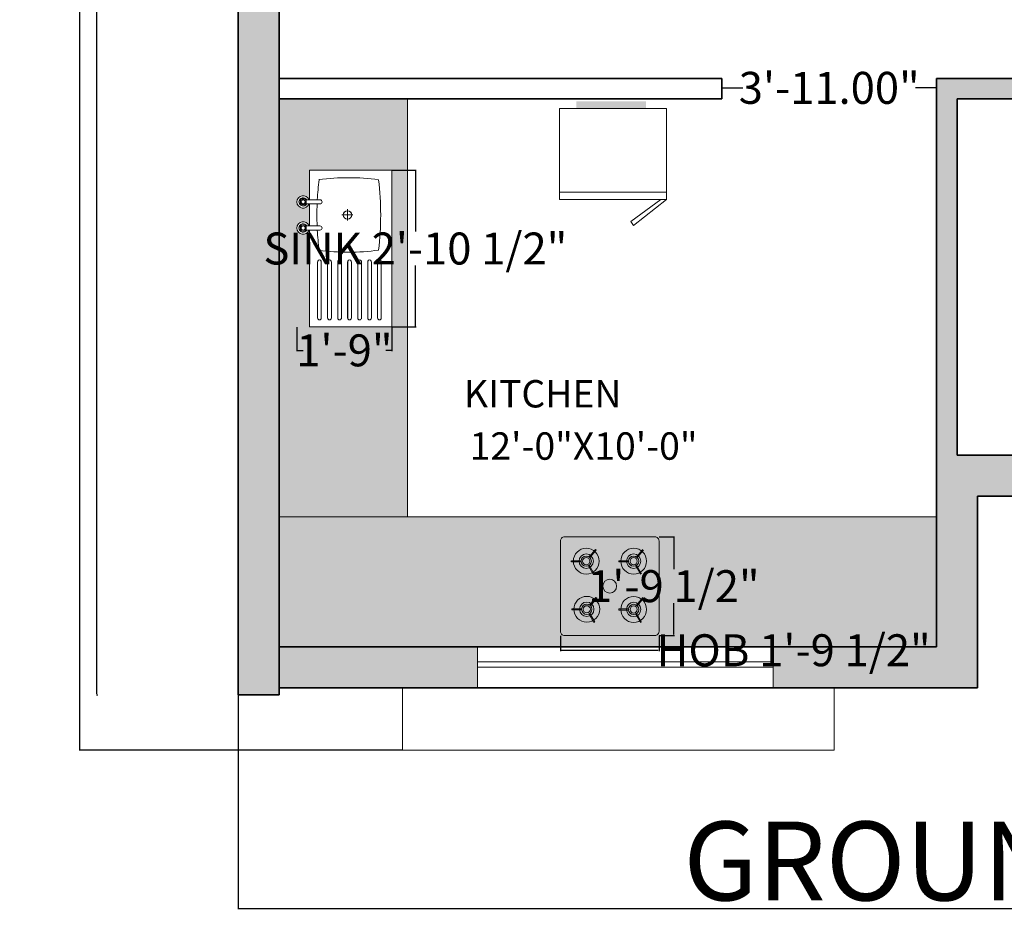
# Model space of a CAD drawing. Units: inches. Extents: x 136 to 672, y -412 to 279.
# Tile 1 of 6: x 136 to 351, y -412 to -213. Entities that reach past the tile are written whole.
import ezdxf

# ---------------------------------------------------------------- set-up
doc = ezdxf.new("R2010")
doc.units = ezdxf.units.IN
doc.header["$MEASUREMENT"] = 0
for name, color, linetype, lineweight in [('A-ANNO-DIMS', 12, 'Continuous', 18), ('A-ANNO-TEXT', 7, 'Continuous', 18), ('A-AREA-IDEN', 7, 'Continuous', 18), ('A-EQPM', 8, 'Continuous', 18), ('A-EQPM-PATT', 252, 'Continuous', 9), ('A-FLOR-CASE', 252, 'Continuous', 18), ('A-FLOR-CASE-PATT', 9, 'Continuous', 9), ('A-FLOR-FIXT', 8, 'Continuous', 18), ('A-FLOR-STRS', 252, 'Continuous', 18), ('A-WALL-PATT', 244, 'Continuous', 9), ('furniture', 252, 'Continuous', 18), ('walls', 253, 'Continuous', 35), ('windows', 171, 'Continuous', 18)]:
    doc.layers.add(name, color=color, linetype=linetype, lineweight=lineweight)
doc.styles.get("Standard").update_dxf_attribs({"font": 'arial.ttf'})
doc.dimstyles.get("Standard").update_dxf_attribs({"dimtxt": 7, "dimasz": 0.18, "dimexe": 0.18, "dimexo": 0.0625, "dimgap": 0.09, "dimtad": 0, "dimtih": 1, "dimtoh": 1, "dimzin": 0, "dimdsep": 46, "dimlunit": 3, "dimtxsty": 'Standard', "dimcen": 0.09, "dimadec": 0, "dimazin": 0, "dimtfac": 1, "dimtofl": 0, "dimtmove": 0, "dimatfit": 3, "dimfxl": 1, "dimtolj": 1, "dimtzin": 0, "dimarcsym": 0})

# ---------------------------------------------------------------- blocks, each defined once
blk = doc.blocks.new('A$C799204C7')
for p, q in [((0, 34.2), (17.99, 34.2)), ((0, 0), (0, 34.2)), ((2.32, 20.01), (2.32, 32.27)), ((3.13, 20.01), (3.13, 32.27)), ((4.48, 20.01), (4.48, 32.27)), ((5.29, 20.01), (5.29, 32.27)), ((6.64, 20.01), (6.64, 32.27)), ((7.45, 20.01), (7.45, 32.27)), ((8.85, 20.01), (8.85, 32.27)), ((9.66, 20.01), (9.66, 32.27)), ((11.01, 20.01), (11.01, 32.27)), ((11.82, 20.01), (11.82, 32.27)), ((13.22, 20.01), (13.22, 32.27)), ((14.03, 20.01), (14.03, 32.27)), ((15.42, 20.01), (15.42, 32.27)), ((16.24, 20.01), (16.24, 32.27)), ((17.99, 13.08), (17.99, 34.2)), ((18.59, 13.08), (15.71, 13.08)), ((9.73, 11), (9.73, 8.54)), ((15.71, 12.17), (18.59, 12.17)), ((17.99, 7.36), (17.99, 12.17)), ((8.52, 9.77), (10.9, 9.77)), ((18.59, 7.36), (15.71, 7.36)), ((15.71, 6.45), (18.59, 6.45)), ((17.99, 0), (17.99, 6.45)), ((0, 0), (17.99, 0))]:
    blk.add_line(p, q)
for centre, radius in [((19.38, 12.62), 0.684), ((19.38, 12.62), 0.456), ((9.7, 9.77), 0.916), ((19.38, 6.91), 0.684), ((19.38, 6.91), 0.456)]:
    blk.add_circle(centre, radius)
for centre, radius, start, end in [((2.72, 32.27), 0.407, 0, 180), ((4.88, 32.27), 0.407, 0, 180), ((7.05, 32.27), 0.407, 0, 180), ((9.25, 32.27), 0.407, 0, 180), ((11.42, 32.27), 0.407, 0, 180), ((13.62, 32.27), 0.407, 0, 180), ((15.83, 32.27), 0.407, 0, 180), ((2.72, 20.01), 0.407, 180, 0), ((4.88, 20.01), 0.407, 180, 0), ((7.05, 20.01), 0.407, 180, 0), ((9.25, 20.01), 0.407, 180, 0), ((11.42, 20.01), 0.407, 180, 0), ((13.62, 20.01), 0.407, 180, 0), ((15.83, 20.01), 0.407, 180, 0), ((67.33, 9.77), 64.88, 173.1952, 186.8048), ((9.53, -30.19), 48.1, 82.3437, 97.8966), ((-48.51, 9.77), 64.88, 2.9208, 6.8048), ((15.71, 12.62), 0.456, 90, 270), ((19.38, 12.62), 1.37, 199.6514, 160.3603), ((19.38, 12.62), 0.911, 210.3431, 149.7554), ((-48.51, 9.77), 64.88, 357.8723, 2.115), ((15.71, 6.91), 0.456, 90, 270), ((-48.51, 9.77), 64.88, 353.1952, 357.0665), ((19.38, 6.91), 1.37, 199.6514, 160.3603), ((19.38, 6.91), 0.911, 210.3431, 149.7554), ((9.53, 49.73), 48.1, 262.1034, 277.6563)]:
    blk.add_arc(centre, radius, start, end)
blk = doc.blocks.new('sink')
at = {"layer": 'furniture'}
for p, q in [((8718164203.894819, -1433730582.369047), (8718164201.504578, -1433730582.369047)), ((8718164202.684322, -1433730581.131674), (8718164202.684322, -1433730583.598095)), ((8718164196.150837, -1433730592.638258), (8718164196.150837, -1433730604.938997)), ((8718164196.967728, -1433730592.638258), (8718164196.967728, -1433730604.938997)), ((8718164198.365185, -1433730592.638258), (8718164198.365185, -1433730604.938997)), ((8718164199.182076, -1433730592.638258), (8718164199.182076, -1433730604.938997)), ((8718164200.579533, -1433730592.638258), (8718164200.579533, -1433730604.938997)), ((8718164201.396423, -1433730592.638258), (8718164201.396423, -1433730604.938997)), ((8718164202.748692, -1433730592.638258), (8718164202.748692, -1433730604.938997)), ((8718164203.565582, -1433730592.638258), (8718164203.565582, -1433730604.938997)), ((8718164204.963041, -1433730592.638258), (8718164204.963041, -1433730604.938997)), ((8718164205.779934, -1433730592.638258), (8718164205.779934, -1433730604.938997)), ((8718164207.1322, -1433730592.638258), (8718164207.1322, -1433730604.938997)), ((8718164207.949093, -1433730592.638258), (8718164207.949093, -1433730604.938997)), ((8718164209.301359, -1433730592.638258), (8718164209.301359, -1433730604.938997)), ((8718164210.118252, -1433730592.638258), (8718164210.118252, -1433730604.938997))]:
    blk.add_line(p, q, dxfattribs=at)
for centre, radius in [((8718164192.998869, -1433730579.495552), 0.685789), ((8718164192.998869, -1433730579.495552), 0.457192), ((8718164202.715019, -1433730582.369047), 0.919003), ((8718164192.998869, -1433730585.228166), 0.68579), ((8718164192.998869, -1433730585.228166), 0.68579), ((8718164192.998869, -1433730585.228166), 0.457192)]:
    blk.add_circle(centre, radius, dxfattribs=at)
for centre, radius, start, end in [((8718164196.559284, -1433730592.638258), 0.41045, 354.3355999, 185.6644001), ((8718164198.77363, -1433730592.638258), 0.41045, 354.3355999, 185.6644001), ((8718164200.98798, -1433730592.638258), 0.41045, 354.3355999, 185.6644001), ((8718164203.157139, -1433730592.638258), 0.41045, 354.3355999, 185.6644001), ((8718164205.371487, -1433730592.638258), 0.41045, 354.3355999, 185.6644001), ((8718164207.540646, -1433730592.640262), 0.41045, 354.3355999, 185.6644001), ((8718164209.709805, -1433730592.640262), 0.41045, 354.3355999, 185.6644001), ((8718164196.559284, -1433730604.938997), 0.408445, 180, 0), ((8718164198.77363, -1433730604.938997), 0.408445, 180, 0), ((8718164200.98798, -1433730604.938997), 0.408445, 180, 0), ((8718164203.157139, -1433730604.938997), 0.408445, 180, 0), ((8718164205.371487, -1433730604.938997), 0.408445, 180, 0), ((8718164207.540646, -1433730604.938997), 0.408445, 180, 0), ((8718164209.709805, -1433730604.938997), 0.408445, 180, 0)]:
    blk.add_arc(centre, radius, start, end, dxfattribs=at)
at = {"layer": 'furniture', "xscale": 1.0032, "yscale": 1.0032, "zscale": 1.0032, "rotation": 180}
blk.add_blockref('A$C799204C7', (8718164212.441259, -1433730572.566334), dxfattribs=at)
blk = doc.blocks.new('washbasin')
at = {"layer": 'furniture'}
blk.add_blockref('sink', (-8718164214.119328, 1433730589.721069), dxfattribs=at)
blk = doc.blocks.new('4bstove')
at = {"layer": 'furniture'}
for p, q in [((1452.73, 1446.21), (1452.73, 1448.61)), ((1452.98, 1446.22), (1452.98, 1448.61)), ((1464.44, 1446.34), (1464.44, 1448.73)), ((1464.69, 1446.34), (1464.69, 1448.73)), ((1451.74, 1444.45), (1449.67, 1443.25)), ((1451.87, 1444.23), (1449.79, 1443.04)), ((1453.75, 1444.08), (1455.58, 1442.54)), ((1453.91, 1444.27), (1455.74, 1442.73)), ((1463.45, 1444.58), (1461.38, 1443.38)), ((1463.57, 1444.36), (1461.5, 1443.17)), ((1465.46, 1444.21), (1467.29, 1442.67)), ((1465.62, 1444.4), (1467.45, 1442.86)), ((1452.69, 1434.81), (1452.69, 1437.2)), ((1452.94, 1434.81), (1452.94, 1437.2)), ((1464.44, 1434.81), (1464.44, 1437.2)), ((1464.69, 1434.81), (1464.69, 1437.2)), ((1451.7, 1433.04), (1449.63, 1431.85)), ((1451.82, 1432.83), (1449.75, 1431.63)), ((1453.71, 1432.67), (1455.54, 1431.13)), ((1453.87, 1432.86), (1455.7, 1431.33)), ((1463.45, 1433.04), (1461.38, 1431.85)), ((1463.57, 1432.83), (1461.5, 1431.63)), ((1465.46, 1432.67), (1467.29, 1431.13)), ((1465.62, 1432.86), (1467.45, 1431.33))]:
    blk.add_line(p, q, dxfattribs=at)
for points in [[(1447.5, 1427.38), (1469.5, 1427.38, 0.414214), (1470.5, 1428.38), (1470.5, 1450.38, 0.414214), (1469.5, 1451.38), (1447.5, 1451.38, 0.414214), (1446.5, 1450.38), (1446.5, 1428.38, 0.414214)], [(1453.75, 1444.97, 1), (1452, 1444.97, 1)], [(1465.46, 1445.1, 1), (1463.71, 1445.1, 1)], [(1453.71, 1433.56, 1), (1451.96, 1433.56, 1)], [(1465.46, 1433.56, 1), (1463.71, 1433.56, 1)]]:
    blk.add_lwpolyline(points, format="xyb", close=True, dxfattribs=at)
for points in [[(1454.12, 1444.97, 1), (1451.62, 1444.97, 1), (1454.12, 1444.97, 1)], [(1465.83, 1445.1, 1), (1463.33, 1445.1, 1), (1465.83, 1445.1, 1)], [(1454.08, 1433.56, 1), (1451.58, 1433.56, 1), (1454.08, 1433.56, 1)], [(1465.83, 1433.56, 1), (1463.33, 1433.56, 1), (1465.83, 1433.56, 1)]]:
    blk.add_lwpolyline(points, format="xyb", dxfattribs=at)
for centre, radius in [((1452.87, 1444.97), 3.14), ((1464.58, 1445.1), 3.14), ((1452.87, 1444.97), 1.75), ((1464.58, 1445.1), 1.75), ((1458.5, 1439.38), 1.67), ((1452.83, 1433.56), 3.14), ((1464.58, 1433.56), 3.14), ((1452.83, 1433.56), 1.75), ((1464.58, 1433.56), 1.75)]:
    blk.add_circle(centre, radius, dxfattribs=at)
for centre, start, end in [((1452.87, 1444.97), 88.2645, 92.2039), ((1464.58, 1445.1), 88.2645, 92.2039), ((1452.87, 1444.97), 208.188, 212.1274), ((1464.58, 1445.1), 208.188, 212.1274), ((1464.58, 1445.1), 318.1018, 322.0412), ((1452.87, 1444.97), 318.1018, 322.0412), ((1452.83, 1433.56), 88.2645, 92.2039), ((1464.58, 1433.56), 88.2645, 92.2039)]:
    blk.add_arc(centre, 3.64, start, end, dxfattribs=at)
blk = doc.blocks.new('stove')
at = {"layer": 'furniture', "xscale": 0.9, "yscale": 0.9, "zscale": 0.9, "rotation": 89.99999999999999}
blk.add_blockref('4bstove', (1295.44, -1312.65), dxfattribs=at)
blk = doc.blocks.new('*D17')
at = {"layer": 'A-ANNO-DIMS', "color": 0, "lineweight": -2, "transparency": 16777216}
for p, q in [((289.46, -226.53), (289.46, -227.69)), ((289.64, -227.51), (294.05, -227.51)), ((336.28, -227.51), (331.87, -227.51)), ((336.46, -226.53), (336.46, -227.69))]:
    blk.add_line(p, q, dxfattribs=at)
at = {"layer": 'A-ANNO-DIMS', "color": 0, "transparency": 16777216}
for points in [[(289.64, -227.48), (289.64, -227.54), (289.46, -227.51)], [(336.28, -227.48), (336.28, -227.54), (336.46, -227.51)]]:
    blk.add_solid(points, dxfattribs=at)
at = {"layer": 'Defpoints', "color": 0, "transparency": 16777216}
for p in [(289.46, -226.47), (336.46, -226.47), (336.46, -227.51)]:
    blk.add_point(p, dxfattribs=at)
at = {"layer": 'A-ANNO-DIMS', "color": 0, "transparency": 16777216, "insert": (312.96, -227.51), "char_height": 7, "attachment_point": 5}
blk.add_mtext('\\A1;3\'-11.00"', dxfattribs=at)
blk = doc.blocks.new('*D19')
at = {"layer": 'A-ANNO-DIMS', "color": 0, "lineweight": -2, "transparency": 16777216}
for p, q in [((152.44, 239.56), (152.7, 239.56)), ((152.52, 239.38), (152.52, -56.77)), ((152.52, -360.26), (152.52, -64.1)), ((152.44, -360.44), (152.7, -360.44))]:
    blk.add_line(p, q, dxfattribs=at)
at = {"layer": 'A-ANNO-DIMS', "color": 0, "transparency": 16777216}
for points in [[(152.49, 239.38), (152.55, 239.38), (152.52, 239.56)], [(152.49, -360.26), (152.55, -360.26), (152.52, -360.44)]]:
    blk.add_solid(points, dxfattribs=at)
at = {"layer": 'Defpoints', "color": 0, "transparency": 16777216}
for p in [(152.38, 239.56), (152.38, -360.44), (152.52, -360.44)]:
    blk.add_point(p, dxfattribs=at)
at = {"layer": 'A-ANNO-DIMS', "color": 0, "transparency": 16777216, "insert": (152.52, -60.44), "char_height": 7, "attachment_point": 5}
blk.add_mtext("\\A1;50'", dxfattribs=at)
blk = doc.blocks.new('*D41')
at = {"layer": 'A-ANNO-DIMS', "color": 0, "lineweight": -2, "transparency": 16777216}
for p, q in [((217.22, -245.55), (222.48, -245.55)), ((222.3, -245.73), (222.3, -259)), ((222.3, -279.68), (222.3, -266.41)), ((217.22, -279.86), (222.48, -279.86))]:
    blk.add_line(p, q, dxfattribs=at)
at = {"layer": 'A-ANNO-DIMS', "color": 0, "transparency": 16777216}
for points in [[(222.27, -245.73), (222.33, -245.73), (222.3, -245.55)], [(222.27, -279.68), (222.33, -279.68), (222.3, -279.86)]]:
    blk.add_solid(points, dxfattribs=at)
at = {"layer": 'Defpoints', "color": 0, "transparency": 16777216}
for p in [(217.16, -245.55), (222.3, -245.55), (217.16, -279.86)]:
    blk.add_point(p, dxfattribs=at)
at = {"layer": 'A-ANNO-DIMS', "color": 0, "transparency": 16777216, "insert": (222.3, -262.7), "char_height": 7, "attachment_point": 5}
blk.add_mtext('\\A1;SINK 2\'-10 1/2"', dxfattribs=at)
blk = doc.blocks.new('*D42')
at = {"layer": 'A-ANNO-DIMS', "color": 0, "lineweight": -2, "transparency": 16777216}
for p, q in [((196.34, -279.92), (196.34, -285.19)), ((217.16, -279.92), (217.16, -285.19)), ((196.52, -285.01), (197.68, -285.01)), ((216.98, -285.01), (215.81, -285.01))]:
    blk.add_line(p, q, dxfattribs=at)
at = {"layer": 'A-ANNO-DIMS', "color": 0, "transparency": 16777216}
for points in [[(196.52, -284.98), (196.52, -285.04), (196.34, -285.01)], [(216.98, -284.98), (216.98, -285.04), (217.16, -285.01)]]:
    blk.add_solid(points, dxfattribs=at)
at = {"layer": 'Defpoints', "color": 0, "transparency": 16777216}
for p in [(196.34, -279.86), (217.16, -279.86), (217.16, -285.01)]:
    blk.add_point(p, dxfattribs=at)
at = {"layer": 'A-ANNO-DIMS', "color": 0, "transparency": 16777216, "insert": (206.75, -285.01), "char_height": 7, "attachment_point": 5}
blk.add_mtext('\\A1;1\'-9"', dxfattribs=at)
blk = doc.blocks.new('*D43')
at = {"layer": 'A-ANNO-DIMS', "color": 0, "lineweight": -2, "transparency": 16777216}
for p, q in [((254.08, -347.52), (254.08, -350.88)), ((275.68, -347.52), (275.68, -350.88)), ((254.26, -350.7), (275.5, -350.7)), ((275.68, -350.7), (275.86, -350.7))]:
    blk.add_line(p, q, dxfattribs=at)
at = {"layer": 'A-ANNO-DIMS', "color": 0, "transparency": 16777216}
for points in [[(254.26, -350.67), (254.26, -350.73), (254.08, -350.7)], [(275.5, -350.67), (275.5, -350.73), (275.68, -350.7)]]:
    blk.add_solid(points, dxfattribs=at)
at = {"layer": 'Defpoints', "color": 0, "transparency": 16777216}
for p in [(254.08, -347.46), (275.68, -347.46), (275.68, -350.7)]:
    blk.add_point(p, dxfattribs=at)
at = {"layer": 'A-ANNO-DIMS', "color": 0, "transparency": 16777216, "insert": (305.18, -350.7), "char_height": 7, "attachment_point": 5}
blk.add_mtext('\\A1;HOB 1\'-9 1/2"', dxfattribs=at)
blk = doc.blocks.new('*D44')
at = {"layer": 'A-ANNO-DIMS', "color": 0, "lineweight": -2, "transparency": 16777216}
for p, q in [((275.74, -325.86), (279.1, -325.86)), ((278.92, -326.04), (278.92, -332.95)), ((278.92, -347.28), (278.92, -340.37)), ((275.74, -347.46), (279.1, -347.46))]:
    blk.add_line(p, q, dxfattribs=at)
at = {"layer": 'A-ANNO-DIMS', "color": 0, "transparency": 16777216}
for points in [[(278.89, -326.04), (278.95, -326.04), (278.92, -325.86)], [(278.89, -347.28), (278.95, -347.28), (278.92, -347.46)]]:
    blk.add_solid(points, dxfattribs=at)
at = {"layer": 'Defpoints', "color": 0, "transparency": 16777216}
for p in [(275.68, -325.86), (278.92, -325.86), (275.68, -347.46)]:
    blk.add_point(p, dxfattribs=at)
at = {"layer": 'A-ANNO-DIMS', "color": 0, "transparency": 16777216, "insert": (278.92, -336.66), "char_height": 7, "attachment_point": 5}
blk.add_mtext('\\A1;1\'-9 1/2"', dxfattribs=at)
blk = doc.blocks.new('*D55')
at = {"layer": 'A-ANNO-DIMS', "color": 0, "lineweight": -2, "transparency": 16777216}
for p, q in [((626.7, -359.5), (626.7, -407.41)), ((183.46, -360.5), (183.46, -407.41)), ((183.64, -407.23), (390.25, -407.23)), ((626.52, -407.23), (419.91, -407.23))]:
    blk.add_line(p, q, dxfattribs=at)
at = {"layer": 'A-ANNO-DIMS', "color": 0, "transparency": 16777216}
for points in [[(183.64, -407.2), (183.64, -407.26), (183.46, -407.23)], [(626.52, -407.2), (626.52, -407.26), (626.7, -407.23)]]:
    blk.add_solid(points, dxfattribs=at)
at = {"layer": 'Defpoints', "color": 0, "transparency": 16777216}
for p in [(626.7, -359.44), (183.46, -360.44), (626.7, -407.23)]:
    blk.add_point(p, dxfattribs=at)
at = {"layer": 'A-ANNO-DIMS', "color": 0, "transparency": 16777216, "insert": (405.08, -407.23), "char_height": 7, "attachment_point": 5}
blk.add_mtext('\\A1;36\'-11"', dxfattribs=at)
blk = doc.blocks.new('*D56')
at = {"layer": 'A-ANNO-DIMS', "color": 0, "lineweight": -2, "transparency": 16777216}
for p, q in [((183.4, 239.56), (148.63, 239.56)), ((148.81, 239.38), (148.81, -62.84)), ((148.81, -372.4), (148.81, -70.17)), ((219.39, -372.58), (148.63, -372.58))]:
    blk.add_line(p, q, dxfattribs=at)
at = {"layer": 'A-ANNO-DIMS', "color": 0, "transparency": 16777216}
for points in [[(148.78, 239.38), (148.84, 239.38), (148.81, 239.56)], [(148.78, -372.4), (148.84, -372.4), (148.81, -372.58)]]:
    blk.add_solid(points, dxfattribs=at)
at = {"layer": 'Defpoints', "color": 0, "transparency": 16777216}
for p in [(183.46, 239.56), (148.81, -372.58), (219.45, -372.58)]:
    blk.add_point(p, dxfattribs=at)
at = {"layer": 'A-ANNO-DIMS', "color": 0, "transparency": 16777216, "insert": (148.81, -66.51), "char_height": 7, "attachment_point": 5}
blk.add_mtext('\\A1;51\'-0"', dxfattribs=at)

msp = doc.modelspace()

# ---------------------------------------------------------------- hatches: boundary and pattern name
at = {"layer": 'A-EQPM-PATT'}
h = msp.add_hatch(color=256, dxfattribs=at)
h.dxf.hatch_style = 1
h.paths.add_polyline_path([(257.594, -230.47), (257.594, -232.035), (272.826, -232.035), (272.826, -230.47)])
at = {"layer": 'A-FLOR-CASE-PATT'}
h = msp.add_hatch(color=256, dxfattribs=at)
h.dxf.hatch_style = 1
h.paths.add_polyline_path([(220.586, -229.935), (192.463, -229.935), (192.463, -321.463), (220.586, -321.463)])
h.paths.add_polyline_path([(199.106, -279.859), (199.106, -258.669), (199.006, -258.669, -5.8284271), (199.006, -257.754), (199.106, -257.754), (199.106, -252.936), (199.006, -252.936, -5.8284271), (199.006, -252.022), (199.106, -252.022), (199.106, -245.55), (217.155, -245.55), (217.155, -279.859)], flags=16)
h.paths.add_polyline_path([(211.846, -277.923), (211.846, -265.622), (211.846, -265.622), (211.846, -265.664, -0.9999793), (212.663, -265.583), (212.663, -277.922, -0.9987905)], flags=0)
h.paths.add_polyline_path([(209.677, -277.923), (209.677, -265.622), (209.677, -265.622), (209.677, -265.662, -0.9999835), (210.494, -265.581), (210.494, -277.922, -0.9988816)], flags=0)
h.paths.add_polyline_path([(214.016, -277.924), (214.016, -265.622), (214.016, -265.622), (214.016, -265.664, -0.999975), (214.832, -265.583), (214.832, -277.922, -0.9987059)], flags=0)
h.paths.add_polyline_path([(207.463, -277.922), (207.463, -265.622, -1), (208.28, -265.622), (208.28, -277.922, -1)], flags=0)
h.paths.add_polyline_path([(207.463, -277.922), (207.463, -265.662, -0.9999765), (208.28, -265.581), (208.28, -277.922, -1)], flags=0)
h.paths.add_polyline_path([(205.294, -277.922), (205.294, -265.622, -1), (206.111, -265.622), (206.111, -277.922, -1)], flags=0)
h.paths.add_polyline_path([(205.294, -277.922), (205.294, -265.662, -0.9999765), (206.111, -265.581), (206.111, -277.922, -1)], flags=0)
h.paths.add_polyline_path([(203.896, -265.581), (203.896, -277.922), (203.896, -277.922), (203.896, -277.922, -1), (203.079, -277.922), (203.079, -277.922, 1.0002364), (203.896, -277.922), (203.896, -265.622, 1.0006671), (203.079, -265.622), (203.079, -265.662, -1)], flags=0)
h.paths.add_polyline_path([(200.865, -277.922), (200.865, -277.922, 1), (201.682, -277.922), (201.682, -277.922, -1.0009232)], flags=0)
h.paths.add_polyline_path([(201.682, -265.622, 1.0013689), (200.865, -265.623), (200.865, -265.662, -1), (201.682, -265.581)], flags=0)
h.paths.add_polyline_path([(207.399, -256.271, -0.4044615), (206.51, -255.353), (206.51, -255.353, 0.4044617), (207.399, -256.271), (207.399, -255.353), (206.51, -255.353, 0.4044615), (207.399, -256.271), (207.399, -256.271, -0.4044619), (206.51, -255.353), (206.219, -255.353), (206.219, -255.353), (206.51, -255.353, -0.404462), (207.399, -254.434), (207.399, -254.115), (207.399, -254.115), (207.399, -254.434, -0.4240325), (208.348, -255.353), (208.348, -255.353, 0.4240328), (207.399, -254.434), (207.399, -255.353), (208.348, -255.353, 0.4240325), (207.399, -254.434), (207.399, -254.434, -0.4240328), (208.348, -255.353), (208.609, -255.353), (208.609, -255.353), (208.348, -255.353, -0.4240329), (207.399, -256.271), (207.399, -256.582), (207.399, -256.582)], flags=0)
h.paths.add_polyline_path([(198.399, -258.212, -1), (197.027, -258.212, -1)], flags=0)
h.paths.add_polyline_path([(198.17, -258.212, -1), (197.256, -258.212, -1)], flags=0)
h.paths.add_polyline_path([(198.399, -252.479, -1), (197.027, -252.479, -1)], flags=0)
h.paths.add_polyline_path([(198.17, -252.479, -1), (197.256, -252.479, -1)], flags=0)
h.paths.add_polyline_path([(336.463, -321.463), (192.463, -321.463), (192.463, -349.935), (336.463, -349.935)])
at = {"layer": 'A-WALL-PATT'}
h = msp.add_hatch(color=256, dxfattribs=at)
h.dxf.hatch_style = 1
h.paths.add_polyline_path([(255.026, 239.565), (183.463, 239.565), (183.463, 125.252), (187.963, 125.252), (192.463, 125.252), (192.463, 230.565), (255.024, 230.565), (255.025, 235.065)])
h.paths.add_polyline_path([(369.355, 239.565), (332.259, 239.565), (332.259, 230.565), (342.463, 230.565), (342.463, 104.521), (346.963, 104.521), (346.963, 230.565), (369.355, 230.565), (369.355, 235.065)])
h.paths.add_polyline_path([(603.463, 239.565), (385.627, 239.565), (385.627, 230.565), (406.963, 230.565), (406.963, 134.565), (371.802, 134.565), (371.802, 130.065), (406.963, 130.065), (406.963, 45.565), (346.963, 45.565), (346.963, 69.395), (342.463, 69.395), (342.463, 45.565), (332.733, 45.565), (332.733, 41.065), (416.87, 41.065), (416.87, 45.565), (411.463, 45.565), (411.463, 230.565), (594.463, 230.565), (594.463, 199.893), (598.963, 199.893), (603.463, 199.893)])
h.paths.add_polyline_path([(603.463, 145.845), (594.463, 145.845), (594.463, 98.065), (524.374, 98.065), (512.275, 97.948), (512.275, 98.065), (484.021, 98.065), (484.021, 93.565), (505.963, 93.565), (594.463, 93.565), (594.463, 80.073), (598.963, 80.073), (603.463, 80.073)], flags=17)
h.paths.add_polyline_path([(457.963, 98.065), (453.463, 98.065), (453.463, 41.065), (594.463, 41.065), (594.463, -67.933), (603.463, -67.933), (603.463, 63.801), (594.463, 63.801), (594.463, 45.565), (510.463, 45.565), (510.463, 65.243), (505.963, 65.243), (505.963, 45.565), (457.963, 45.565)])
h.paths.add_polyline_path([(192.463, 71.205), (183.463, 71.205), (183.463, 25.824), (192.463, 25.824), (192.463, 41.065), (296.463, 41.065), (296.463, 24.884), (300.963, 24.884), (300.963, 45.565), (192.463, 45.565)])
h.paths.add_polyline_path([(300.963, -6.935), (296.463, -6.935), (192.463, -6.935), (192.463, -11.435), (300.963, -11.435)])
h.paths.add_polyline_path([(192.463, 8.674), (183.463, 8.674), (183.463, -44.733), (187.963, -44.733), (192.463, -44.733)])
h.paths.add_polyline_path([(235.886, -349.935), (192.463, -349.935), (192.463, -358.935), (235.886, -358.935)])
h.paths.add_polyline_path([(345.463, -316.935), (361.986, -316.935), (361.986, -307.935), (340.963, -307.935), (340.963, -229.935), (356.354, -229.935), (356.354, -225.435), (336.463, -225.435), (336.463, -349.935), (300.655, -349.935), (300.655, -358.935), (345.463, -358.935)])
h.paths.add_polyline_path([(407.452, -307.935), (403.463, -307.935), (403.463, -225.435), (382.286, -225.435), (382.286, -229.935), (398.963, -229.935), (398.963, -307.935), (379.137, -307.935), (379.137, -316.935), (407.452, -316.935)])
h.paths.add_polyline_path([(470.463, -284.28), (461.463, -284.28), (461.463, -307.935), (461.463, -316.935), (470.463, -316.935)])
h.paths.add_polyline_path([(470.463, -234.435), (480.349, -234.435), (480.349, -225.435), (461.463, -225.435), (461.463, -245.135), (470.463, -245.135)])
h.paths.add_polyline_path([(603.463, -121.943), (594.463, -121.943), (594.463, -225.435), (574.368, -225.435), (574.368, -234.435), (603.463, -234.435)])
h.paths.add_polyline_path([(340.963, -75.678), (336.463, -75.678), (336.463, -168.061), (340.963, -168.061)])
h.paths.add_polyline_path([(468.637, 59.14), (510.671, 59.14), (510.671, 68.331), (468.637, 68.331)], flags=25)
h.paths.add_polyline_path([(192.463, -208.04), (183.463, -208.04), (183.463, -360.435), (192.463, -360.435)])
h.paths.add_polyline_path([(183.463, -153.992), (192.463, -153.992), (192.463, -98.781), (183.463, -98.781)])

# ---------------------------------------------------------------- linework, layer by layer
at = {"layer": 'A-EQPM'}
for p, q in [((253.851, -251.96), (253.851, -232.035)), ((253.851, -232.035), (277.315, -232.035)), ((277.315, -232.035), (277.315, -251.96)), ((277.315, -250.366), (253.851, -250.366)), ((277.315, -251.96), (253.851, -251.96)), ((269.513, -256.761), (276.034, -251.96)), ((277.315, -251.96), (270.053, -257.675)), ((270.053, -257.675), (269.513, -256.761))]:
    msp.add_line(p, q, dxfattribs=at)
at = {"layer": 'A-FLOR-CASE'}
for p, q in [((220.586, -229.935), (220.586, -321.463)), ((336.463, -321.463), (192.463, -321.463))]:
    msp.add_line(p, q, dxfattribs=at)
at = {"layer": 'A-FLOR-STRS'}
for p, q in [((219.455, -358.935), (219.455, -372.578)), ((314.058, -372.578), (314.058, -358.935)), ((219.455, -372.578), (314.058, -372.578))]:
    msp.add_line(p, q, dxfattribs=at)
at = {"layer": 'walls'}
for p, q in [((183.463, -360.435), (183.463, 239.565)), ((192.463, -360.435), (192.463, 41.065)), ((192.463, -225.435), (289.463, -225.435)), ((289.463, -227.507), (289.463, -225.435)), ((289.463, -225.435), (289.463, -229.935)), ((336.463, -349.935), (336.463, -225.435)), ((336.463, -225.435), (594.463, -225.435)), ((289.463, -227.507), (289.463, -227.507)), ((192.463, -229.935), (289.463, -229.935)), ((340.963, -307.935), (340.963, -229.935)), ((340.963, -229.935), (356.354, -229.935)), ((340.963, -307.935), (398.963, -307.935)), ((345.463, -316.935), (470.463, -316.935)), ((345.463, -358.935), (345.463, -316.935)), ((192.463, -349.935), (336.463, -349.935)), ((192.463, -358.935), (345.463, -358.935)), ((192.463, -360.435), (183.463, -360.435))]:
    msp.add_line(p, q, dxfattribs=at)
at = {"layer": 'windows'}
for p, q in [((235.886, -349.935), (235.886, -358.935)), ((300.655, -349.935), (235.886, -349.935)), ((235.886, -349.935), (235.886, -353.236)), ((300.655, -358.935), (300.655, -349.935)), ((235.886, -353.236), (300.655, -353.236)), ((300.655, -353.236), (300.655, -354.435)), ((300.655, -354.435), (235.886, -354.435)), ((235.886, -358.935), (300.655, -358.935))]:
    msp.add_line(p, q, dxfattribs=at)

# ---------------------------------------------------------------- block references
at = {"layer": 'A-EQPM'}
msp.add_blockref('stove', (264.881, -336.657), dxfattribs=at)
at = {"layer": 'A-FLOR-FIXT'}
msp.add_blockref('washbasin', (218.834, -262.705), dxfattribs=at)

# ---------------------------------------------------------------- texts
at = {"layer": 'A-ANNO-TEXT'}
msp.add_text('GROUND FLOOR PLAN', height=17.26909, dxfattribs=at).set_placement((281.023, -405.489))
at = {"layer": 'A-AREA-IDEN'}
for s, p in [('KITCHEN', (232.939, -297.52)), ('12\'-0"X10\'-0"', (234.177, -308.967))]:
    msp.add_text(s, height=6, dxfattribs=at).set_placement(p)

# ---------------------------------------------------------------- dimensions: what is measured, and where the dimension line sits
at = {"layer": 'A-ANNO-DIMS'}
for base, p1, p2, override, picture, middle in [((148.813, -372.578), (183.463, 239.565), (219.455, -372.578), {"dimdec": 1, "dimlfac": 1, "dimrnd": 0, "dimzin": 1, "dimdsep": 46, "dimlunit": 4, "dimfrac": 2}, '*D56', (148.813, -66.506)), ((152.519, -360.435), (152.38, 239.565), (152.38, -360.435), {"dimclrd": 0, "dimclre": 0, "dimclrt": 0}, '*D19', (152.519, -60.435)), ((278.921, -325.857), (275.681, -347.457), (275.681, -325.857), {"dimdec": 1, "dimlfac": 1, "dimrnd": 0, "dimzin": 1, "dimdsep": 46, "dimlunit": 4, "dimfrac": 2}, '*D44', (278.921, -336.657))]:
    dim = msp.add_linear_dim(base=base, p1=p1, p2=p2, angle=90, dimstyle='Standard', override=override, dxfattribs=at)
    dim.commit()
    dim.dimension.update_dxf_attribs({"geometry": picture, "text_midpoint": middle})
for base, p1, p2, override, picture, middle in [((336.463, -227.507), (289.463, -226.471), (336.463, -226.471), {"dimclrd": 0, "dimclre": 0, "dimclrt": 0}, '*D17', (312.963, -227.507)), ((217.155, -285.006), (196.341, -279.859), (217.155, -279.859), {"dimdec": 1, "dimlfac": 1, "dimrnd": 0, "dimzin": 1, "dimdsep": 46, "dimlunit": 4, "dimfrac": 2}, '*D42', (206.748, -285.006)), ((626.698, -407.228), (183.463, -360.435), (626.698, -359.435), {"dimdec": 1, "dimlfac": 1, "dimrnd": 0, "dimzin": 1, "dimdsep": 46, "dimlunit": 4, "dimfrac": 2}, '*D55', (405.08, -407.228))]:
    dim = msp.add_linear_dim(base=base, p1=p1, p2=p2, dimstyle='Standard', override=override, dxfattribs=at)
    dim.commit()
    dim.dimension.update_dxf_attribs({"geometry": picture, "text_midpoint": middle})
dim = msp.add_linear_dim(base=(222.302, -245.55), p1=(217.155, -279.859), p2=(217.155, -245.55), angle=90, text='SINK <>', dimstyle='Standard', override={"dimdec": 1, "dimlfac": 1, "dimrnd": 0, "dimzin": 1, "dimdsep": 46, "dimlunit": 4, "dimfrac": 2}, dxfattribs=at)
dim.commit()
dim.dimension.update_dxf_attribs({"geometry": '*D41', "text_midpoint": (222.302, -262.705)})
dim = msp.add_linear_dim(base=(275.681, -350.697), p1=(254.081, -347.457), p2=(275.681, -347.457), text='HOB <>', dimstyle='Standard', override={"dimdec": 1, "dimlfac": 1, "dimrnd": 0, "dimzin": 1, "dimdsep": 46, "dimlunit": 4, "dimfrac": 2}, dxfattribs=at)
dim.commit()
dim.dimension.update_dxf_attribs({"geometry": '*D43', "text_midpoint": (305.176, -350.697)})

doc.saveas('drawing.dxf')
